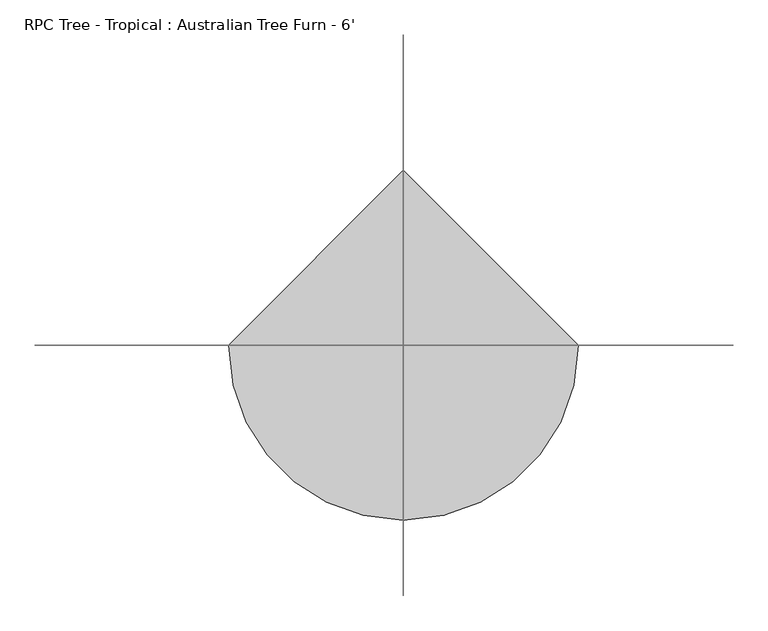
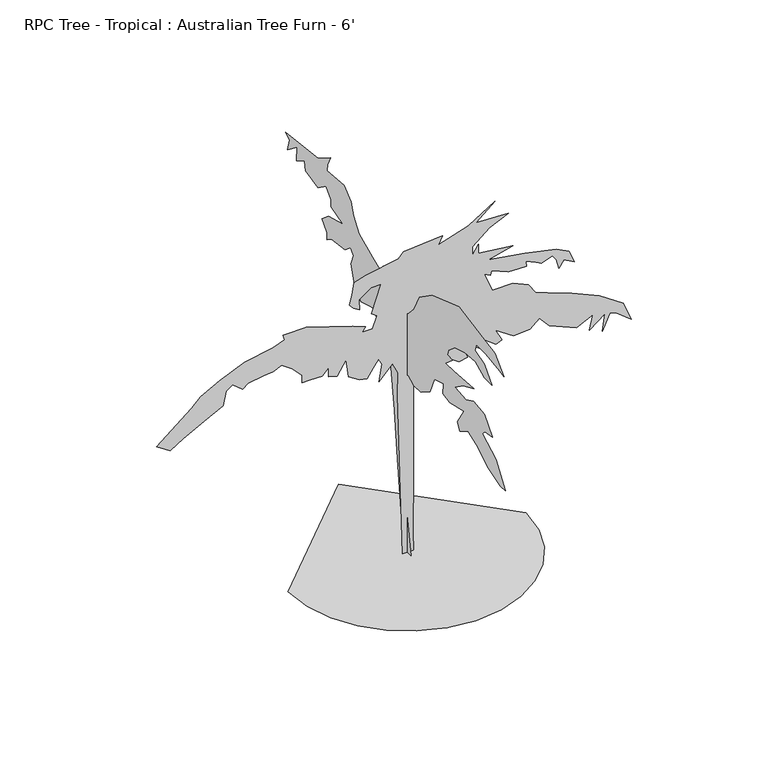
"""IFC4 building model written with IfcOpenShell, lengths in millimetres: geographic element geometry, RPC Tree - Tropical : Australian Tree Furn - 6'."""

from ifc_helpers import new_model, si_unit, origin, place, context, project, spatial, triangles, source, transform, mapped, element, save


def rpc_tree_tropical_australian_tree_furn_6_77f1a640(model_context):
    return source(origin(), model_context, "Body", "Tessellation", [
        triangles([(-639.0365753, 0.0, 0.0007159), (-622.1405136, -146.4247652, 0.0007159), (-574.0277527, -280.8912123, 0.0007159), (-498.5465315, -399.5499215, 0.0007159), (-399.5499215, -498.5465315, 0.0007159), (-280.8912123, -574.0277527, 0.0007159), (-146.4247652, -622.1405136, 0.0007159), (2.79e-05, -639.0365753, 0.0007159), (146.4247652, -622.1429844, 0.0007159), (280.8912123, -574.0277527, 0.0007159), (399.5499215, -498.5465315, 0.0007159), (498.5465315, -399.5499215, 0.0007159), (574.0277527, -280.8912123, 0.0007159), (622.1405136, -146.4247652, 0.0007159), (639.0365753, 5.59e-05, 0.0007159), (-8.38e-05, 639.0365753, 0.0007159), (470.2991641, -3.5e-05, 1828.8014534), (368.5593713, -2.98e-05, 1741.5955845), (542.9711454, -2.94e-05, 1734.3285862), (441.231389, -2.66e-05, 1687.0922253), (350.3907492, -2.2e-05, 1610.7880165), (350.3907492, -1.92e-05, 1563.5516556), (383.0932589, -2.22e-05, 1614.4202076), (383.0932589, -1.92e-05, 1563.5516556), (568.4067295, -1.79e-05, 1541.750806), (437.5966181, -1.59e-05, 1509.0482964), (633.8092781, -1.4e-05, 1476.3456413), (800.9540903, -1.18e-05, 1440.0109406), (869.9913008, -9.7e-06, 1403.673769), (899.0591486, -5.5e-06, 1334.6364132), (840.9235256, -7.5e-06, 1367.3389229), (815.4879416, -5.1e-06, 1327.3695602), (800.9540903, -8.4e-06, 1381.8729195), (779.1532408, -1.01e-05, 1410.9406219), (721.015147, -8.8e-06, 1389.1397724), (691.9473719, -9.7e-06, 1403.673769), (637.4440126, -1.12e-05, 1429.1092804), (641.0762037, -9.4e-06, 1400.0414326), (597.4745047, -9.4e-06, 1400.0414326), (542.9711454, -9.7e-06, 1403.673769), (452.1330491, -1.18e-05, 1440.0109406), (448.4983146, -1.03e-05, 1414.5754292), (415.7958049, -1.14e-05, 1432.7440876), (459.4000111, -5.1e-06, 1327.3695602), (568.4067295, -5.1e-06, 1327.3695602), (651.9778639, -2.9e-06, 1291.0347141), (688.3126373, 3e-07, 1236.5313549), (753.7176567, 1.8e-06, 1211.0958435), (884.5252247, 4.9e-06, 1160.2246754), (1033.5014511, 8.7e-06, 1094.8221268), (1160.6767553, 1.39e-05, 1007.6162579), (1204.2784544, 2.02e-05, 902.2417305), (1120.70732, 1.63e-05, 967.6468225), (1088.0048103, 1.59e-05, 974.9137482), (1048.0353024, 2.11e-05, 887.7078793), (1062.5692263, 1.55e-05, 982.1806738), (978.9980919, 1.94e-05, 916.7781979), (997.1666777, 1.44e-05, 1000.3493322), (909.9608088, 1.7e-05, 956.7450897), (764.6193169, 1.33e-05, 1018.5179907), (710.1159576, 9.6e-06, 1080.2882755), (659.2448622, 1.22e-05, 1036.684033), (572.0389206, 1.26e-05, 1029.4171074), (473.9338986, 8.7e-06, 1094.8221268), (510.2686357, 1.26e-05, 1029.4171074), (477.5660897, 1.35e-05, 1014.8831835), (324.9577085, 6.6e-06, 1131.1569002), (419.4305394, 1.44e-05, 1000.3493322), (284.9882369, 8.7e-06, 1094.8221268), (324.9577085, 1.48e-05, 993.0824066), (277.7212749, 1.52e-05, 985.8154083), (190.5151335, 1.16e-05, 1047.5857658), (88.7756132, 9.6e-06, 1080.2882755), (194.1488688, 1.52e-05, 985.8154083), (30.6385209, 1.11e-05, 1054.8526915), (34.2719928, 1.57e-05, 978.5484827), (34.2719928, 3.32e-05, 684.2282936), (34.2719928, 4.84e-05, 429.8801196), (30.6385209, 6.77e-05, 106.4923825), (34.2719928, 7.35e-05, 0.0013276), (-23.8650472, 7.39e-05, 0.0007003), (-52.9336422, 1.98e-05, 909.5111996), (-49.2999159, 1.22e-05, 1036.684033), (-78.3684632, 8.5e-06, 1098.4543905), (-151.0396997, 1.31e-05, 1022.1501818), (-136.5055487, 7.5e-06, 1116.6229763), (-154.6734259, 5.5e-06, 1149.325486), (-183.7417098, 7.9e-06, 1109.3560507), (-216.4437289, 1.07e-05, 1062.1196171), (-256.4132006, 1.03e-05, 1069.3865427), (-314.5512943, 8.1e-06, 1105.7213161), (-329.0852182, 2e-06, 1207.461109), (-376.3216155, 6.6e-06, 1131.1569002), (-423.5580491, 5.7e-06, 1145.6907515), (-423.5580491, 2.7e-06, 1196.5619196), (-456.2580153, 4.9e-06, 1160.2246754), (-518.0283365, 4.9e-06, 1160.2246754), (-565.2647701, 4.9e-06, 1160.2246754), (-565.2647701, 2.3e-06, 1203.8289179), (-619.7706728, -1e-06, 1258.3322044), (-674.2714886, -3.4e-06, 1298.3017124), (-721.5079222, -2.1e-06, 1276.5008629), (-772.3790903, -1.9e-06, 1272.866201), (-855.9502247, -1e-06, 1258.3322044), (-885.0205433, 3e-07, 1236.5313549), (-939.5239025, -2.3e-06, 1280.133054), (-972.2238688, -8e-07, 1254.6975426), (-990.3925272, 3.8e-06, 1178.3933338), (-1092.13232, 6.8e-06, 1127.5247091), (-1204.773773, 1.05e-05, 1065.7543516), (-1273.8110561, 1.31e-05, 1022.1501818), (-1346.4830738, 1.03e-05, 1069.3865427), (-1157.5373394, 1.2e-06, 1221.9975037), (-1110.3009058, -1.9e-06, 1272.866201), (-1008.561113, -5.1e-06, 1327.3695602), (-874.1188105, -8.6e-06, 1385.5075813), (-721.5079222, -1.03e-05, 1414.5754292), (-659.7375647, -1.16e-05, 1436.3762787), (-667.004563, -1.33e-05, 1465.4439812), (-539.8317295, -1.33e-05, 1465.4439812), (-416.2885437, -1.1e-05, 1425.4770893), (-292.7479377, -8.6e-06, 1385.5075813), (-223.7109271, -7.1e-06, 1360.0720699), (-241.8788043, -5.5e-06, 1334.6364132), (-187.3751907, -5.5e-06, 1334.6364132), (-161.9403697, -9.4e-06, 1400.0414326), (-191.0089079, -1.07e-05, 1421.8422821), (-140.1390206, -1.96e-05, 1570.8185085), (-194.6423889, -1.96e-05, 1570.8185085), (-260.0454098, -1.68e-05, 1523.5821476), (-256.4132006, -1.33e-05, 1465.4439812), (-289.1157284, -1.46e-05, 1487.2474468), (-310.9165598, -1.62e-05, 1512.6804874), (-296.3826722, -1.94e-05, 1567.1838467), (-285.4809939, -2.31e-05, 1628.956675), (-220.0774642, -2.44e-05, 1650.7575245), (-45.666444, -2.63e-05, 1683.4600342), (-20.2313959, -2.81e-05, 1712.5277367), (190.5151335, -2.92e-05, 1730.6963951), (168.7137935, -2.66e-05, 1687.0922253), (328.5898996, -2.96e-05, 1737.9633934), (3.03e-05, -861.8582216, 1549.8330162), (2.4e-05, -733.5424347, 1570.5289913), (2.01e-05, -646.6209961, 1570.5289913), (2.06e-05, -630.0627771, 1529.1370411), (2.54e-05, -721.12437, 1504.3009117), (3.07e-05, -787.3523769, 1425.6574562), (2.76e-05, -716.9866865, 1425.6574562), (2.26e-05, -634.2029314, 1467.0492611), (1.86e-05, -539.0011479, 1458.7689526), (1.52e-05, -443.8018716, 1429.7951397), (1.41e-05, -385.8542459, 1380.1253517), (1.46e-05, -373.4361812, 1347.0113846), (1.68e-05, -423.1059328, 1347.0113846), (1.55e-05, -356.8778895, 1289.0637589), (1.89e-05, -435.5239975, 1293.2039131), (2.69e-05, -621.7848667, 1305.6220505), (2.36e-05, -518.3052092, 1260.089946), (2.19e-05, -443.8018716, 1206.2800037), (2.68e-05, -547.2815291, 1198.0020933), (2.89e-05, -617.6471832, 1231.1161331), (3.37e-05, -716.9866865, 1218.6980684), (3.97e-05, -795.6302147, 1135.9143133), (3.69e-05, -725.2645243, 1123.4987921), (3.66e-05, -700.4309383, 1098.6626627), (4.42e-05, -824.6040276, 1028.2969723), (5.2e-05, -915.6656204, 904.1213396), (4.99e-05, -865.9959051, 899.9836561), (4.34e-05, -745.9604994, 937.2353794), (3.69e-05, -642.4808418, 999.3231594), (3.26e-05, -567.9774679, 1032.4371992), (3.06e-05, -489.3313963, 982.7648678), (2.84e-05, -468.6354575, 1024.1567453), (2.82e-05, -530.7232738, 1123.4987921), (2.33e-05, -398.2697671, 1090.3847523), (2e-05, -332.0443036, 1102.802817), (1.84e-05, -336.1819871, 1160.7504427), (1.55e-05, -253.3997399, 1135.9143133), (1.65e-05, -212.0081348, 1040.715037), (1.44e-05, -129.2246341, 986.9050947), (1.15e-05, -62.9981487, 982.7648678), (8.4e-06, -13.3280768, 1011.7412241), (6.8e-06, 32.2026538, 999.3231594), (4.5e-06, 52.8985925, 1044.8527205), (4.9e-06, 81.8726461, 986.9050947), (7e-06, 86.0118375, 912.3991774), (1.57e-05, 57.0377794, 664.0505281), (2.77e-05, 19.7852431, 316.3597959), (3.93e-05, -34.0238362, 0.0007149), (3.64e-05, 36.3418406, 0.0), (3.07e-05, 52.8985925, 167.3503229), (1.97e-05, 90.1512742, 477.7870791), (1.08e-05, 119.1250779, 734.4162186), (1.5e-06, 156.3777732, 991.0453217), (-4.8e-06, 210.1869524, 1119.3585651), (-7.3e-06, 268.135323, 1119.3585651), (-1.14e-05, 305.3869918, 1198.0020933), (-1.38e-05, 371.6149987, 1181.4464178), (-1.58e-05, 429.5625881, 1160.7504427), (-2.04e-05, 491.6504045, 1222.8382954), (-2.47e-05, 520.6242173, 1322.177726), (-2.55e-05, 499.9282785, 1380.1253517), (-2.76e-05, 528.9020914, 1409.0991646), (-2.86e-05, 578.5718067, 1367.7072144), (-3.37e-05, 702.7474394, 1351.1515388), (-3.47e-05, 744.1393169, 1322.177726), (-3.59e-05, 744.1393169, 1363.5696762), (-3.96e-05, 793.8090322, 1413.2393188), (-3.83e-05, 731.7212523, 1462.9091068), (-3.35e-05, 599.2677455, 1500.1607574), (-3.93e-05, 706.8876663, 1533.2747246), (-4.06e-05, 711.0252771, 1570.5289913), (-4.41e-05, 756.5573816, 1620.1987793), (-4.58e-05, 831.0607555, 1566.3888371), (-5.18e-05, 946.9584778, 1591.2223503), (-5.36e-05, 955.2363155, 1640.8946091), (-5.57e-05, 1029.7422329, 1599.5028042), (-5.79e-05, 1025.602006, 1678.1462597), (-5.98e-05, 1112.525988, 1611.9183254), (-6.09e-05, 1095.9676964, 1674.0061054), (-6.33e-05, 1133.2218904, 1698.8422348), (-5.08e-05, 831.0607555, 1731.9562019), (-4.78e-05, 715.1655041, 1806.4596485), (-4.73e-05, 739.99909, 1752.652177), (-4.64e-05, 748.2795439, 1711.2603722), (-3.97e-05, 586.8496808, 1727.8160477), (-3.52e-05, 520.6242173, 1674.0061054), (-3.23e-05, 499.9282785, 1607.7806419), (-2.78e-05, 446.1183363, 1537.4150242), (-2.05e-05, 321.9452471, 1479.4647823), (-1.04e-05, 143.960199, 1409.0991646), (-1.65e-05, 226.7434454, 1487.7452362), (-9.7e-06, 114.9858956, 1429.7951397), (-2.2e-06, -0.9105653, 1351.1515388), (-1.4e-06, -62.9981487, 1417.3796185), (-2.2e-06, -112.668141, 1516.7190491), (7e-07, -232.7038011, 1599.5028042), (9.2e-06, -481.0535222, 1686.4242428), (2.03e-05, -700.4309383, 1645.0322926), (2.61e-05, -816.3261898, 1624.3363174), (3.23e-05, -899.1099449, 1541.5525623)], [[15, 16, 1], [14, 15, 1], [14, 1, 2], [13, 14, 2], [13, 2, 3], [13, 3, 4], [12, 13, 4], [11, 12, 4], [11, 4, 5], [11, 5, 6], [11, 6, 7], [11, 7, 8], [11, 8, 9], [11, 9, 10], [141, 17, 18], [54, 55, 56], [73, 74, 75], [67, 68, 69], [24, 25, 26], [18, 19, 20], [51, 52, 53], [22, 23, 24], [84, 85, 86], [29, 30, 31], [56, 57, 58], [31, 32, 33], [130, 131, 132], [138, 139, 140], [41, 42, 43], [111, 112, 113], [110, 111, 113], [109, 110, 113], [122, 123, 124], [118, 119, 120], [18, 20, 21], [141, 18, 21], [69, 70, 71], [69, 71, 72], [28, 29, 31], [28, 31, 33], [28, 33, 34], [27, 28, 34], [27, 34, 35], [27, 35, 36], [27, 36, 37], [130, 132, 133], [130, 133, 134], [50, 51, 53], [50, 53, 54], [50, 54, 56], [50, 56, 58], [140, 141, 21], [37, 38, 39], [64, 65, 66], [64, 66, 67], [80, 81, 82], [79, 80, 82], [78, 79, 82], [77, 78, 82], [76, 77, 82], [76, 82, 83], [75, 76, 83], [97, 98, 99], [49, 50, 58], [49, 58, 59], [49, 59, 60], [48, 49, 60], [48, 60, 61], [47, 48, 61], [129, 130, 134], [129, 134, 135], [129, 135, 136], [129, 136, 137], [128, 129, 137], [108, 109, 113], [108, 113, 114], [107, 108, 114], [107, 114, 115], [106, 107, 115], [106, 115, 116], [105, 106, 116], [104, 105, 116], [103, 104, 116], [103, 116, 117], [102, 103, 117], [101, 102, 117], [101, 117, 118], [75, 83, 84], [26, 27, 37], [26, 37, 39], [26, 39, 40], [26, 40, 41], [26, 41, 43], [92, 93, 94], [92, 94, 95], [126, 127, 128], [101, 118, 120], [100, 101, 120], [100, 120, 121], [99, 100, 121], [97, 99, 121], [96, 97, 121], [95, 96, 121], [95, 121, 122], [92, 95, 122], [92, 122, 124], [140, 21, 22], [88, 89, 90], [24, 26, 43], [22, 24, 43], [88, 90, 91], [88, 91, 92], [88, 92, 124], [87, 88, 124], [87, 124, 125], [47, 61, 62], [47, 62, 63], [47, 63, 64], [46, 47, 64], [45, 46, 64], [44, 45, 64], [44, 64, 67], [43, 44, 67], [137, 138, 140], [128, 137, 140], [126, 128, 140], [126, 140, 22], [126, 22, 43], [126, 43, 67], [126, 67, 69], [126, 69, 72], [126, 72, 73], [125, 126, 73], [87, 125, 73], [87, 73, 75], [87, 75, 84], [87, 84, 86], [231, 232, 233], [156, 157, 158], [240, 241, 142], [222, 223, 224], [218, 219, 220], [220, 221, 222], [218, 220, 222], [153, 154, 155], [240, 142, 143], [239, 240, 143], [146, 147, 148], [205, 206, 207], [162, 163, 164], [156, 158, 159], [216, 217, 218], [216, 218, 222], [166, 167, 168], [166, 168, 169], [222, 224, 225], [239, 143, 144], [238, 239, 144], [146, 148, 149], [145, 146, 149], [165, 166, 169], [165, 169, 170], [207, 208, 209], [188, 189, 190], [188, 190, 191], [188, 191, 192], [187, 188, 192], [187, 192, 193], [186, 187, 193], [186, 193, 194], [185, 186, 194], [171, 172, 173], [171, 173, 174], [145, 149, 150], [155, 156, 159], [165, 170, 171], [165, 171, 174], [175, 176, 177], [182, 183, 184], [205, 207, 209], [205, 209, 210], [204, 205, 210], [203, 204, 210], [161, 162, 164], [161, 164, 165], [161, 165, 174], [160, 161, 174], [159, 160, 174], [159, 174, 175], [159, 175, 177], [155, 159, 177], [238, 144, 145], [238, 145, 150], [237, 238, 150], [237, 150, 151], [237, 151, 152], [236, 237, 152], [235, 236, 152], [235, 152, 153], [235, 153, 155], [235, 155, 177], [235, 177, 178], [234, 235, 178], [234, 178, 179], [234, 179, 180], [234, 180, 181], [234, 181, 182], [234, 182, 184], [231, 233, 234], [231, 234, 184], [214, 215, 216], [214, 216, 222], [213, 214, 222], [213, 222, 225], [213, 225, 226], [212, 213, 226], [212, 226, 227], [212, 227, 228], [211, 212, 228], [210, 211, 228], [210, 228, 229], [203, 210, 229], [203, 229, 230], [202, 203, 230], [184, 185, 194], [184, 194, 195], [231, 184, 195], [230, 231, 195], [230, 195, 196], [230, 196, 197], [202, 230, 197], [202, 197, 198], [201, 202, 198], [200, 201, 198], [199, 200, 198]], closed=False),
    ])


if __name__ == "__main__":
    model = new_model("IFC4")
    model_context = context("Model", 3, world=origin())
    ifc_project = project(units=[si_unit("LENGTHUNIT", "METRE", prefix="MILLI")], contexts=[model_context])
    site = spatial("IfcSite", under=ifc_project)
    building = spatial("IfcBuilding", under=site)
    placement = place(None, origin())
    rpc_tree_tropical_australian_tree_furn_6_shape = rpc_tree_tropical_australian_tree_furn_6_77f1a640(model_context)
    element("IfcGeographicElement", 1, ObjectType="RPC Tree - Tropical : Australian Tree Furn - 6'", at=placement, inside=building, context=model_context, shape_type="MappedRepresentation", body=[
        mapped(rpc_tree_tropical_australian_tree_furn_6_shape, transform((0.0, 0.0, 0.0), x_axis=(1.0, 0.0, 0.0), y_axis=(0.0, 1.0, 0.0), z_axis=(0.0, 0.0, 1.0))),
    ])
    save(model, "model.ifc")

# Revit data of these elements
# Type "RPC Tree - Tropical : Australian Tree Furn - 6'"
#   built-in parameter 1005198 = "{2, 15},{39, RPC-16-FVCN-UWG0-AP53-A000-ST1L-LVER-AU},{1, 0},{1, 0},{2, 13},{1, 8},{5, Color},{1, 0},{1, 0},{3, 0.8},{3, 0.8},{3, 0.8},{1, 8},{7, BBoxMin},{1, 0},{1, 0},{1, 0},{1, 0},{1, 0},{1, 8},{7, BBoxMax},{1, 0},{1, 0},{1, 0},{1, 0},{1, 0},{2, 11},{9, RPCTypeId},{1, 0},{1, 0},{39, RPC-16-FVCN-UWG0-AP53-A000-ST1L-LVER-AU},{1, 6},{14, RPCPlantHeight},{1, 0},{1, 0},{1, 6},{2, 11},{7, keyword},{1, 0},{1, 0},{35, :RPCs:Trees [Tropical]:Geometry:RPC},{2, 11},{8, category},{1, 0},{1, 0},{16, Trees [Tropical]},{2, 11},{12, LocalizedUID},{1, 0},{1, 0},{20, Australian Tree Fern},{2, 14},{6, Height},{1, 0},{1, 0},{1, 6},{1, 2},{16, Cast Reflections},{1, 0},{1, 0},{1, 0},{1, 2},{12, Cast Shadows},{1, 0},{1, 0},{1, 1},{1, 2},{9, Lock View},{1, 0},{1, 0},{1, 0},{1, 4},{5, ViewC},{1, 0},{1, 0},{1, 0},{21, assetlibrary_base.fbx},{1, 5},"
#   built-in parameter 1005195 = "RPC-16-FVCN-UWG0-AP53-A000-ST1L-LVER-AU"
#   Type Comments = "Australian Tree Furn"
#   Assembly Code = "G2050500"
#   Height = 6' - 0"
#   Plan Symbol = element 363555
#   Default Elevation = 0
